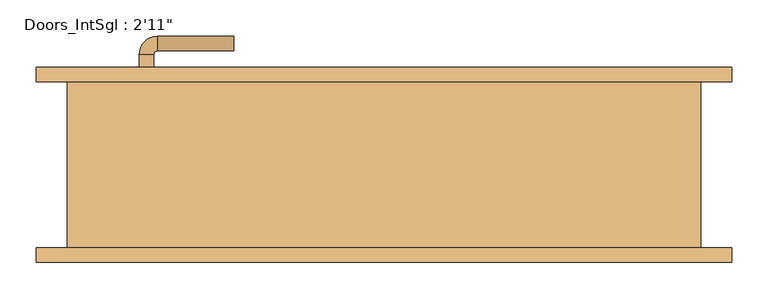
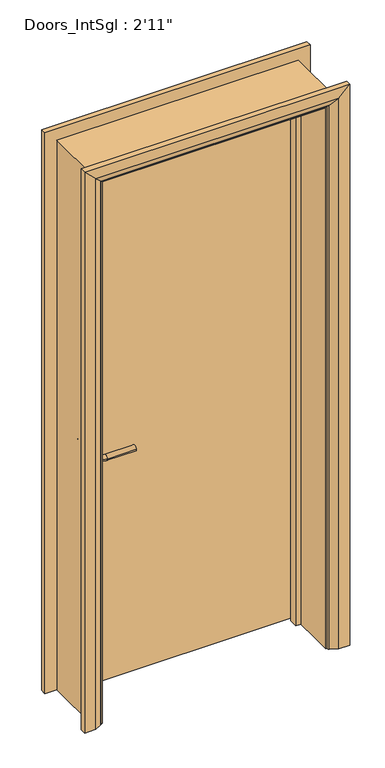
"""IFC4 building model written with IfcOpenShell, lengths in millimetres: door geometry."""

from ifc_helpers import new_model, si_unit, point, frame, frame_2d, origin, place, context, project, spatial, polyline, circle_curve, ellipse_curve, trimmed, segment, composite_curve, outline, extrude, faceted_brep, source, transform, mapped, element, save
from ifc_brep_helpers import plane_surface, cylinder_surface, revolved_surface, advanced_brep


def door_61435f0d(model_context):
    return source(origin(), model_context, "Body", "SolidModel", [
        advanced_brep(
        [(-337.5, 68.3, 900.0), (-317.5, 68.3, 900.0), (-317.5, 38.3, 900.0), (-337.5, 38.3, 900.0), (-312.5, 33.3, 900.0), (-312.5, 13.3, 900.0), (-207.5, 13.3, 900.0), (-207.5, 33.3, 900.0)],
        [
            (0, 1, circle_curve(frame((-327.5, 68.3, 900.0), z_axis=(0.0, 1.0, 0.0), x_axis=(1.0, 0.0, 0.0)), 10.0)),
            (1, 0, circle_curve(frame((-327.5, 68.3, 900.0), z_axis=(0.0, 1.0, 0.0), x_axis=(1.0, 0.0, 0.0)), 10.0)),
            (1, 2),
            (2, 3, circle_curve(frame((-327.5, 38.3, 900.0), z_axis=(0.0, 1.0, 0.0), x_axis=(1.0, 0.0, 0.0)), 10.0)),
            (3, 0),
            (3, 2, circle_curve(frame((-327.5, 38.3, 900.0), z_axis=(0.0, 1.0, 0.0), x_axis=(1.0, 0.0, 0.0)), 10.0)),
            (4, 5, circle_curve(frame((-312.5, 23.3, 900.0), z_axis=(-1.0, 0.0, 0.0), x_axis=(0.0, 1.0, 0.0)), 10.0)),
            (5, 3, circle_curve(frame((-312.5, 38.3, 900.0), z_axis=(0.0, 0.0, -1.0), x_axis=(-1.0, 0.0, 0.0)), 25.0)),
            (2, 4, circle_curve(frame((-312.5, 38.3, 900.0), z_axis=(0.0, 0.0, 1.0), x_axis=(-1.0, 0.0, 0.0)), 5.0)),
            (5, 4, circle_curve(frame((-312.5, 23.3, 900.0), z_axis=(-1.0, 0.0, 0.0), x_axis=(0.0, 1.0, 0.0)), 10.0)),
            (6, 7, circle_curve(frame((-207.5, 23.3, 900.0), z_axis=(1.0, 0.0, 0.0), x_axis=(0.0, 1.0, 0.0)), 10.0)),
            (7, 6, circle_curve(frame((-207.5, 23.3, 900.0), z_axis=(1.0, 0.0, 0.0), x_axis=(0.0, 1.0, 0.0)), 10.0)),
            (4, 7),
            (6, 5),
        ],
        [
            plane_surface(frame((-327.5, 68.3, 900.0), z_axis=(0.0, 1.0, 0.0), x_axis=(0.0, 0.0, 1.0))),
            cylinder_surface(frame((-327.5, 68.3, 900.0), z_axis=(0.0, 1.0, 0.0), x_axis=(1.0, 0.0, 0.0)), 10.0),
            revolved_surface(trimmed(ellipse_curve(frame((-327.5, 38.3, 900.0), z_axis=(0.0, -1.0, 0.0), x_axis=(1.0, 0.0, 0.0)), 10.0, 10.0), [point((-337.5, 38.3, 900.0))], [point((-317.5, 38.3, 900.0))], True, "CARTESIAN"), (-312.5, 38.3, 900.0), (0.0, 0.0, -1.0)),
            revolved_surface(trimmed(ellipse_curve(frame((-327.5, 38.3, 900.0), z_axis=(0.0, -1.0, 0.0), x_axis=(1.0, 0.0, 0.0)), 10.0, 10.0), [point((-317.5, 38.3, 900.0))], [point((-337.5, 38.3, 900.0))], True, "CARTESIAN"), (-312.5, 38.3, 900.0), (0.0, 0.0, -1.0)),
            plane_surface(frame((-207.5, 23.3, 900.0), z_axis=(1.0, 0.0, 0.0), x_axis=(0.0, 0.0, 1.0))),
            cylinder_surface(frame((-312.5, 23.3, 900.0), z_axis=(-1.0, 0.0, 0.0), x_axis=(0.0, 1.0, 0.0)), 10.0),
        ],
        [
            (0, [[1, 2]]),
            (1, [[3, 4, 5, -2]]),
            (1, [[-5, 6, -3, -1]]),
            (2, [[7, 8, -4, 9]]),
            (3, [[10, -9, -6, -8]]),
            (4, [[11, 12]]),
            (5, [[13, -11, 14, -7]]),
            (5, [[-14, -12, -13, -10]]),
        ],
    ),
        extrude(outline(composite_curve([segment(trimmed(circle_curve(frame_2d((900.0, -330.0)), 30.0), [point((900.0, -360.0))], [point((900.0, -300.0))], False, "CARTESIAN"), True, "CONTINUOUS"), segment(trimmed(circle_curve(frame_2d((900.0, -330.0)), 30.0), [point((900.0, -300.0))], [point((900.0, -360.0))], False, "CARTESIAN"), True, "CONTINUOUS")], self_intersect=False)), frame((0.0, 68.3, 0.0), z_axis=(0.0, 1.0, 0.0), x_axis=(0.0, 0.0, 1.0)), (0.0, 0.0, 1.0), 8.0),
        advanced_brep(
        [(-337.5, 122.3, 900.0), (-317.5, 122.3, 900.0), (-337.5, 152.3, 900.0), (-317.5, 152.3, 900.0), (-312.5, 157.3, 900.0), (-312.5, 177.3, 900.0), (-207.5, 177.3, 900.0), (-207.5, 157.3, 900.0)],
        [
            (0, 1, circle_curve(frame((-327.5, 122.3, 900.0), z_axis=(0.0, -1.0, 0.0), x_axis=(1.0, 0.0, 0.0)), 10.0)),
            (1, 0, circle_curve(frame((-327.5, 122.3, 900.0), z_axis=(0.0, -1.0, 0.0), x_axis=(1.0, 0.0, 0.0)), 10.0)),
            (0, 2),
            (2, 3, circle_curve(frame((-327.5, 152.3, 900.0), z_axis=(0.0, -1.0, 0.0), x_axis=(1.0, 0.0, 0.0)), 10.0)),
            (3, 1),
            (3, 2, circle_curve(frame((-327.5, 152.3, 900.0), z_axis=(0.0, -1.0, 0.0), x_axis=(1.0, 0.0, 0.0)), 10.0)),
            (4, 3, circle_curve(frame((-312.5, 152.3, 900.0), z_axis=(0.0, 0.0, 1.0), x_axis=(-1.0, 0.0, 0.0)), 5.0)),
            (2, 5, circle_curve(frame((-312.5, 152.3, 900.0), z_axis=(0.0, 0.0, -1.0), x_axis=(-1.0, 0.0, 0.0)), 25.0)),
            (5, 4, circle_curve(frame((-312.5, 167.3, 900.0), z_axis=(-1.0, 0.0, 0.0), x_axis=(0.0, -1.0, 0.0)), 10.0)),
            (4, 5, circle_curve(frame((-312.5, 167.3, 900.0), z_axis=(-1.0, 0.0, 0.0), x_axis=(0.0, -1.0, 0.0)), 10.0)),
            (6, 7, circle_curve(frame((-207.5, 167.3, 900.0), z_axis=(1.0, 0.0, 0.0), x_axis=(0.0, -1.0, 0.0)), 10.0)),
            (7, 6, circle_curve(frame((-207.5, 167.3, 900.0), z_axis=(1.0, 0.0, 0.0), x_axis=(0.0, -1.0, 0.0)), 10.0)),
            (5, 6),
            (7, 4),
        ],
        [
            plane_surface(frame((-327.5, 122.3, 900.0), z_axis=(0.0, -1.0, 0.0), x_axis=(0.0, 0.0, 1.0))),
            cylinder_surface(frame((-327.5, 122.3, 900.0), z_axis=(0.0, -1.0, 0.0), x_axis=(1.0, 0.0, 0.0)), 10.0),
            revolved_surface(trimmed(ellipse_curve(frame((-327.5, 152.3, 900.0), z_axis=(0.0, -1.0, 0.0), x_axis=(1.0, 0.0, 0.0)), 10.0, 10.0), [point((-337.5, 152.3, 900.0))], [point((-317.5, 152.3, 900.0))], True, "CARTESIAN"), (-312.5, 152.3, 900.0), (0.0, 0.0, -1.0)),
            revolved_surface(trimmed(ellipse_curve(frame((-327.5, 152.3, 900.0), z_axis=(0.0, -1.0, 0.0), x_axis=(1.0, 0.0, 0.0)), 10.0, 10.0), [point((-317.5, 152.3, 900.0))], [point((-337.5, 152.3, 900.0))], True, "CARTESIAN"), (-312.5, 152.3, 900.0), (0.0, 0.0, -1.0)),
            plane_surface(frame((-207.5, 167.3, 900.0), z_axis=(1.0, 0.0, 0.0), x_axis=(0.0, 0.0, 1.0))),
            cylinder_surface(frame((-312.5, 167.3, 900.0), z_axis=(-1.0, 0.0, 0.0), x_axis=(0.0, -1.0, 0.0)), 10.0),
        ],
        [
            (0, [[1, 2]]),
            (1, [[-1, 3, 4, 5]]),
            (1, [[-2, -5, 6, -3]]),
            (2, [[7, -4, 8, 9]]),
            (3, [[-8, -6, -7, 10]]),
            (4, [[11, 12]]),
            (5, [[-9, 13, -12, 14]]),
            (5, [[-10, -14, -11, -13]]),
        ],
    ),
        extrude(outline(composite_curve([segment(trimmed(circle_curve(frame_2d((900.0, -330.0)), 30.0), [point((900.0, -360.0))], [point((900.0, -300.0))], False, "CARTESIAN"), True, "CONTINUOUS"), segment(trimmed(circle_curve(frame_2d((900.0, -330.0)), 30.0), [point((900.0, -300.0))], [point((900.0, -360.0))], False, "CARTESIAN"), True, "CONTINUOUS")], self_intersect=False)), frame((0.0, 114.3, 0.0), z_axis=(0.0, 1.0, 0.0), x_axis=(0.0, 0.0, 1.0)), (0.0, 0.0, 1.0), 8.0),
        extrude(outline(polyline([(402.5, 76.3), (-402.5, 76.3), (-402.5, 114.3), (402.5, 114.3), (402.5, 76.3)])), frame((0.0, 0.0, 8.0), z_axis=(0.0, 0.0, 1.0), x_axis=(1.0, 0.0, 0.0)), (0.0, 0.0, 1.0), 2060.0),
        advanced_brep(
        [(479.5, 134.3, 0.0), (479.5, 114.3, 0.0), (409.5, 114.3, 0.0), (413.5, 120.3, 0.0), (439.5, 134.3, 0.0), (479.5, 134.3, 2145.0), (479.5, 114.3, 2145.0), (-479.5, 114.3, 2145.0), (-479.5, 114.3, 0.0), (-409.5, 114.3, 0.0), (-409.5, 114.3, 2075.0), (409.5, 114.3, 2075.0), (413.5, 120.3, 2079.0), (439.5, 134.3, 2105.0), (-439.5, 134.3, 2105.0), (-439.5, 134.3, 0.0), (-479.5, 134.3, 0.0), (-479.5, 134.3, 2145.0), (-413.5, 120.3, 0.0), (-413.5, 120.3, 2079.0)],
        [
            (0, 1),
            (1, 2),
            (2, 3, circle_curve(frame((417.5, 113.3, 0.0), z_axis=(0.0, 0.0, -1.0), x_axis=(1.0, 0.0, 0.0)), 8.0622577)),
            (3, 4),
            (4, 0),
            (0, 5),
            (5, 6),
            (6, 1),
            (6, 7),
            (7, 8),
            (8, 9),
            (9, 10),
            (10, 11),
            (11, 2),
            (11, 12, ellipse_curve(frame((417.5, 113.3, 2083.0), z_axis=(0.7071067811865475, 0.0, -0.7071067811865475), x_axis=(-0.7071067811865474, 0.0, -0.7071067811865476)), 11.4017543, 8.0622577)),
            (12, 3),
            (12, 13),
            (13, 4),
            (13, 14),
            (14, 15),
            (15, 16),
            (16, 17),
            (17, 5),
            (7, 17),
            (16, 8),
            (15, 18),
            (18, 9, circle_curve(frame((-417.5, 113.3, 0.0), z_axis=(0.0, 0.0, -1.0), x_axis=(-1.0, 0.0, 0.0)), 8.0622577)),
            (19, 10, ellipse_curve(frame((-417.5, 113.3, 2083.0), z_axis=(-0.7071067811865475, 0.0, -0.7071067811865475), x_axis=(-0.7071067811865474, 0.0, 0.7071067811865476)), 11.4017543, 8.0622577)),
            (18, 19),
            (14, 19),
            (19, 12),
        ],
        [
            plane_surface(frame((409.5, 114.3, 0.0), z_axis=(0.0, 0.0, -1.0), x_axis=(0.0, -1.0, 0.0))),
            plane_surface(frame((479.5, 134.3, 0.0), z_axis=(1.0, 0.0, 0.0), x_axis=(0.0, 0.0, 1.0))),
            plane_surface(frame((479.5, 114.3, 0.0), z_axis=(0.0, -1.0, 0.0), x_axis=(0.0, 0.0, 1.0))),
            cylinder_surface(frame((417.5, 113.3, 0.0), z_axis=(0.0, 0.0, -1.0), x_axis=(1.0, 0.0, 0.0)), 8.0622577),
            plane_surface(frame((413.5, 120.3, 0.0), z_axis=(-0.4740998230350126, 0.880471099922178, 0.0), x_axis=(0.0, 0.0, 1.0))),
            plane_surface(frame((439.5, 134.3, 0.0), z_axis=(0.0, 1.0, 0.0), x_axis=(0.0, 0.0, 1.0))),
            plane_surface(frame((-479.5, 134.3, 2145.0), z_axis=(-1.0, 0.0, 0.0), x_axis=(0.0, 0.0, -1.0))),
            plane_surface(frame((-409.5, 114.3, 0.0), z_axis=(0.0, 0.0, -1.0), x_axis=(0.0, -1.0, 0.0))),
            cylinder_surface(frame((-417.5, 113.3, 2075.0), z_axis=(0.0, 0.0, 1.0), x_axis=(-1.0, 0.0, 0.0)), 8.0622577),
            plane_surface(frame((-413.5, 120.3, 2079.0), z_axis=(0.47409982303501824, 0.8804710999221749, 0.0), x_axis=(0.0, 0.0, -1.0))),
            plane_surface(frame((479.5, 134.3, 2145.0), z_axis=(0.0, 0.0, 1.0), x_axis=(-1.0, 0.0, 0.0))),
            cylinder_surface(frame((409.5, 113.3, 2083.0), z_axis=(1.0, 0.0, 0.0), x_axis=(0.0, 0.0, 1.0)), 8.0622577),
            plane_surface(frame((413.5, 120.3, 2079.0), z_axis=(0.0, 0.8804710999221764, -0.4740998230350154), x_axis=(-1.0, 0.0, 0.0))),
        ],
        [
            (0, [[1, 2, 3, 4, 5]]),
            (1, [[-1, 6, 7, 8]]),
            (2, [[-2, -8, 9, 10, 11, 12, 13, 14]]),
            (3, [[-3, -14, 15, 16]]),
            (4, [[-4, -16, 17, 18]]),
            (5, [[-5, -18, 19, 20, 21, 22, 23, -6]]),
            (6, [[24, -22, 25, -10]]),
            (7, [[-21, 26, 27, -11, -25]]),
            (8, [[28, -12, -27, 29]]),
            (9, [[30, -29, -26, -20]]),
            (10, [[-7, -23, -24, -9]]),
            (11, [[-15, -13, -28, 31]]),
            (12, [[-17, -31, -30, -19]]),
        ],
    ),
        extrude(outline(polyline([(0.0, -404.5), (0.0, -385.5), (2051.0, -385.5), (2051.0, 385.5), (0.0, 385.5), (0.0, 404.5), (2070.0, 404.5), (2070.0, -404.5), (0.0, -404.5)])), frame((0.0, 42.3, 0.0), z_axis=(0.0, 1.0, 0.0), x_axis=(0.0, 0.0, 1.0)), (0.0, 0.0, 1.0), 32.0),
        advanced_brep(
        [(-479.5, -134.3, 0.0), (-479.5, -114.3, 0.0), (-409.5, -114.3, 0.0), (-413.5, -120.3, 0.0), (-439.5, -134.3, 0.0), (-479.5, -134.3, 2145.0), (-479.5, -114.3, 2145.0), (-409.5, -114.3, 2075.0), (-413.5, -120.3, 2079.0), (-439.5, -134.3, 2105.0), (479.5, -134.3, 0.0), (439.5, -134.3, 0.0), (413.5, -120.3, 0.0), (409.5, -114.3, 0.0), (479.5, -114.3, 0.0), (479.5, -134.3, 2145.0), (439.5, -134.3, 2105.0), (413.5, -120.3, 2079.0), (409.5, -114.3, 2075.0), (479.5, -114.3, 2145.0)],
        [
            (0, 1),
            (1, 2),
            (2, 3, circle_curve(frame((-417.5, -113.3, 0.0), z_axis=(0.0, 0.0, -1.0), x_axis=(-1.0, 0.0, 0.0)), 8.0622577)),
            (3, 4),
            (4, 0),
            (0, 5),
            (5, 6),
            (6, 1),
            (6, 7),
            (7, 2),
            (7, 8, ellipse_curve(frame((-417.5, -113.3, 2083.0), z_axis=(-0.7071067811865475, 0.0, -0.7071067811865475), x_axis=(0.7071067811865474, 0.0, -0.7071067811865476)), 11.4017543, 8.0622577)),
            (8, 3),
            (8, 9),
            (9, 4),
            (9, 5),
            (10, 11),
            (11, 12),
            (12, 13, circle_curve(frame((417.5, -113.3, 0.0), z_axis=(0.0, 0.0, -1.0), x_axis=(1.0, 0.0, 0.0)), 8.0622577)),
            (13, 14),
            (14, 10),
            (15, 16),
            (16, 11),
            (10, 15),
            (16, 17),
            (17, 12),
            (17, 18, ellipse_curve(frame((417.5, -113.3, 2083.0), z_axis=(0.7071067811865475, 0.0, -0.7071067811865475), x_axis=(0.7071067811865474, 0.0, 0.7071067811865476)), 11.4017543, 8.0622577)),
            (18, 13),
            (18, 19),
            (19, 14),
            (19, 15),
            (5, 15),
            (19, 6),
            (18, 7),
            (17, 8),
            (16, 9),
        ],
        [
            plane_surface(frame((-409.5, -187.1010989, 0.0), z_axis=(0.0, 0.0, -1.0), x_axis=(1.0, 0.0, 0.0))),
            plane_surface(frame((-479.5, -134.3, 0.0), z_axis=(-1.0, 0.0, 0.0), x_axis=(0.0, 0.0, 1.0))),
            plane_surface(frame((-479.5, -114.3, 0.0), z_axis=(0.0, 1.0, 0.0), x_axis=(0.0, 0.0, 1.0))),
            cylinder_surface(frame((-417.5, -113.3, 0.0), z_axis=(0.0, 0.0, -1.0), x_axis=(-1.0, 0.0, 0.0)), 8.0622577),
            plane_surface(frame((-413.5, -120.3, 0.0), z_axis=(0.4740998230350183, -0.8804710999221749, 0.0), x_axis=(0.0, 0.0, 1.0))),
            plane_surface(frame((-439.5, -134.3, 0.0), z_axis=(0.0, -1.0, 0.0), x_axis=(0.0, 0.0, 1.0))),
            plane_surface(frame((409.5, -187.1010989, 0.0), z_axis=(0.0, 0.0, -1.0), x_axis=(-1.0, 0.0, 0.0))),
            plane_surface(frame((439.5, -134.3, 2105.0), z_axis=(0.0, -1.0, 0.0), x_axis=(0.0, 0.0, -1.0))),
            plane_surface(frame((413.5, -120.3, 2079.0), z_axis=(-0.4740998230350183, -0.8804710999221749, 0.0), x_axis=(0.0, 0.0, -1.0))),
            cylinder_surface(frame((417.5, -113.3, 2075.0), z_axis=(0.0, 0.0, 1.0), x_axis=(1.0, 0.0, 0.0)), 8.0622577),
            plane_surface(frame((479.5, -114.3, 2145.0), z_axis=(0.0, 1.0, 0.0), x_axis=(0.0, 0.0, -1.0))),
            plane_surface(frame((479.5, -134.3, 2145.0), z_axis=(1.0, 0.0, 0.0), x_axis=(0.0, 0.0, -1.0))),
            plane_surface(frame((-479.5, -134.3, 2145.0), z_axis=(0.0, 0.0, 1.0), x_axis=(1.0, 0.0, 0.0))),
            plane_surface(frame((-479.5, -114.3, 2145.0), z_axis=(0.0, 1.0, 0.0), x_axis=(1.0, 0.0, 0.0))),
            cylinder_surface(frame((-409.5, -113.3, 2083.0), z_axis=(-1.0, 0.0, 0.0), x_axis=(0.0, 0.0, 1.0)), 8.0622577),
            plane_surface(frame((-413.5, -120.3, 2079.0), z_axis=(0.0, -0.8804710999221749, -0.4740998230350183), x_axis=(1.0, 0.0, 0.0))),
            plane_surface(frame((-439.5, -134.3, 2105.0), z_axis=(0.0, -1.0, 0.0), x_axis=(1.0, 0.0, 0.0))),
        ],
        [
            (0, [[1, 2, 3, 4, 5]]),
            (1, [[-1, 6, 7, 8]]),
            (2, [[-2, -8, 9, 10]]),
            (3, [[-3, -10, 11, 12]]),
            (4, [[-4, -12, 13, 14]]),
            (5, [[-5, -14, 15, -6]]),
            (6, [[16, 17, 18, 19, 20]]),
            (7, [[21, 22, -16, 23]]),
            (8, [[24, 25, -17, -22]]),
            (9, [[26, 27, -18, -25]]),
            (10, [[28, 29, -19, -27]]),
            (11, [[30, -23, -20, -29]]),
            (12, [[-7, 31, -30, 32]]),
            (13, [[-9, -32, -28, 33]]),
            (14, [[-11, -33, -26, 34]]),
            (15, [[-13, -34, -24, 35]]),
            (16, [[-15, -35, -21, -31]]),
        ],
    ),
        faceted_brep([(-404.5, 114.3, 0.0), (-404.5, -114.3, 0.0), (-436.5, -114.3, 0.0), (-436.5, 114.3, 0.0), (-404.5, 114.3, 2070.0), (-404.5, -114.3, 2070.0), (-436.5, -114.3, 2102.0), (-436.5, 114.3, 2102.0), (404.5, 114.3, 0.0), (436.5, 114.3, 0.0), (436.5, -114.3, 0.0), (404.5, -114.3, 0.0), (404.5, 114.3, 2070.0), (436.5, 114.3, 2102.0), (436.5, -114.3, 2102.0), (404.5, -114.3, 2070.0)], [[[0, 1, 2, 3]], [[1, 0, 4, 5]], [[2, 1, 5, 6]], [[3, 2, 6, 7]], [[0, 3, 7, 4]], [[8, 9, 10, 11]], [[12, 13, 9, 8]], [[13, 14, 10, 9]], [[14, 15, 11, 10]], [[15, 12, 8, 11]], [[5, 4, 12, 15]], [[6, 5, 15, 14]], [[7, 6, 14, 13]], [[4, 7, 13, 12]]]),
    ])


if __name__ == "__main__":
    model = new_model("IFC4")
    model_context = context("Model", 3, world=origin())
    ifc_project = project(units=[si_unit("LENGTHUNIT", "METRE", prefix="MILLI")], contexts=[model_context])
    site = spatial("IfcSite", under=ifc_project)
    building = spatial("IfcBuilding", under=site)
    placement = place(None, origin())
    door_shape = door_61435f0d(model_context)
    element("IfcDoor", 1, ObjectType="Doors_IntSgl : 2'11\"", at=placement, inside=building, context=model_context, shape_type="MappedRepresentation", body=[
        mapped(door_shape, transform((0.0, 0.0, 0.0), x_axis=(1.0, 0.0, 0.0), y_axis=(0.0, 1.0, 0.0), z_axis=(0.0, 0.0, 1.0))),
    ])
    save(model, "model.ifc")

# Revit data of these elements
# Type "Doors_IntSgl : 2'11\""
#   Type Mark = "48"
#   Type Comments = "Internal Single"
#   Operation = "SingleSwingRight"
#   Manufacturer = "Revit"
#   Keynote = "L20"
#   Description = "Internal Single Door"
#   Analytic Construction = "Metal"
#   UnderCut = 0' - 0.31496"
#   Tolerance = 0' - 0.07874"
#   Thickness = 0' - 1.49606"
#   Thermal Resistance (R) = 0.270117 (m²·K)/W
#   Structural Tolerance = 0' - 0.31496"
#   StopDepth = 0' - 1.25984"
#   Stop Thickness = 0' - 0.74803"
#   Rough Width = 2' - 11"
#   Rough Height = 6' - 11.07087"
#   Height to Top Lock Rail = 3' - 3.37008"
#   Heat Transfer Coefficient (U) = 3.7021 W/(m²·K)
#   Handle Z Distance = 2' - 11.43307"
#   Handle X Distance = 0' - 2.95276"
#   Frame Thickness = 0' - 1.25984"
#   Door Panel Width = 2' - 7.69291"
#   Door Panel Thickness = 0' - 1.49606"
#   Door Panel Offset = 0' - 0"
#   Height = 6' - 11.07087"
#   Width = 2' - 11"
#   Door Panel Height = 6' - 9.10236"
#   Architrave Setback = 0' - 0.19685"
#   Vis - Ironmongery = yes
#   Material Ironmongery = Door - Handle
#   Material Frame = Door - Frame/Mullion (1)
#   Material Door = Door - Panel
#   Material Architrave = Door - Architrave
#   Visual Light Transmittance = 0
#   Solar Heat Gain Coefficient = 0
#   Function = (empty or 0)
#   Wall Closure = (empty or 0)
# Element 1 (IfcDoor, "Doors_IntSgl : 2'11\"")
#   Materials on its faces: "Door - Architrave", "Door - Handle", "Door - Frame/Mullion (1)", "Door - Panel"
# Materials
#   "Door - Handle": colour RGB 0 0 0, transparency 0, Keynote = "P21", Cost = 0
#   "Door - Frame/Mullion (1)": class "Wood", colour RGB 212 179 113, transparency 0, Keynote = "L20", Cost = 0
#   "Door - Panel": class "Wood", colour RGB 210 159 95, transparency 0, Keynote = "L20", Cost = 0
#   "Door - Architrave": class "Wood", colour RGB 154 90 5, transparency 0, Keynote = "P20", Cost = 0
